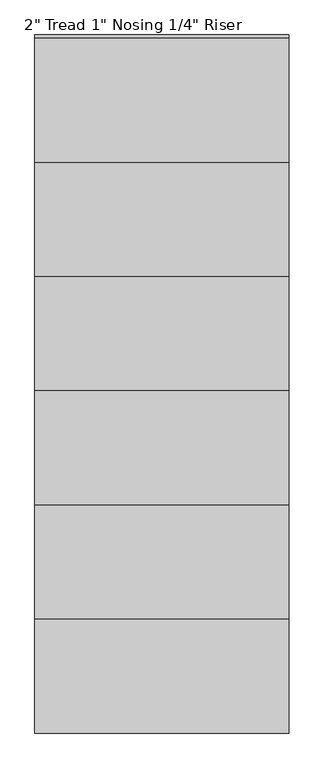
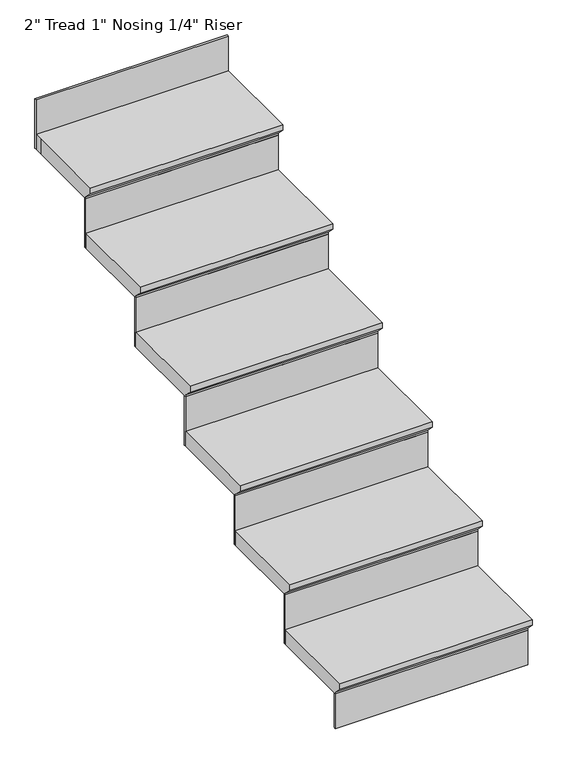
"""IFC4 building model written with IfcOpenShell, lengths in millimetres: stair flight geometry."""

from ifc_helpers import new_model, si_unit, origin, place, context, project, spatial, faceted_brep, source, transform, mapped, element, save


def stair_flight_33de849b(model_context):
    return source(origin(), model_context, "Body", "Brep", [
        faceted_brep([(-912.3629117, -4479.3424149, 150.2833333), (-912.3629117, -4479.3424149, 169.3333333), (-1534.6629117, -4479.3424149, 169.3333333), (-1534.6629117, -4479.3424149, 150.2833333), (-912.3629117, -4453.9424149, 124.8833333), (-1534.6629117, -4453.9424149, 124.8833333), (-912.3629117, -4174.5424149, 169.3333333), (-1534.6629117, -4174.5424149, 169.3333333), (-1534.6629117, -4453.9424149, 118.5333333), (-1534.6629117, -4174.5424149, 118.5333333), (-912.3629117, -4174.5424149, 118.5333333), (-912.3629117, -4453.9424149, 118.5333333)], [[[0, 1, 2, 3]], [[4, 0, 3, 5]], [[2, 1, 6, 7]], [[8, 9, 10, 11]], [[2, 7, 9, 8, 5, 3]], [[8, 11, 4, 5]], [[6, 1, 0, 4, 11, 10]], [[7, 6, 10, 9]]]),
        faceted_brep([(-912.3629117, -4453.9424149, 118.5333333), (-912.3629117, -4453.9424149, 0.0), (-912.3629117, -4447.5924149, 0.0), (-912.3629117, -4447.5924149, 118.5333333), (-1534.6629117, -4453.9424149, 118.5333333), (-1534.6629117, -4447.5924149, 118.5333333), (-1534.6629117, -4447.5924149, 0.0), (-1534.6629117, -4453.9424149, 0.0)], [[[0, 1, 2, 3]], [[4, 5, 6, 7]], [[1, 0, 4, 7]], [[2, 1, 7, 6]], [[3, 2, 6, 5]], [[0, 3, 5, 4]]]),
        faceted_brep([(-912.3629117, -4174.5424149, 287.8666667), (-912.3629117, -4174.5424149, 118.5333333), (-912.3629117, -4168.1924149, 118.5333333), (-912.3629117, -4168.1924149, 287.8666667), (-1534.6629117, -4174.5424149, 287.8666667), (-1534.6629117, -4168.1924149, 287.8666667), (-1534.6629117, -4168.1924149, 118.5333333), (-1534.6629117, -4174.5424149, 118.5333333)], [[[0, 1, 2, 3]], [[4, 5, 6, 7]], [[1, 0, 4, 7]], [[2, 1, 7, 6]], [[3, 2, 6, 5]], [[0, 3, 5, 4]]]),
        faceted_brep([(-1534.6629117, -4199.9424149, 338.6666667), (-912.3629117, -4199.9424149, 338.6666667), (-912.3629117, -3895.1424149, 338.6666667), (-1534.6629117, -3895.1424149, 338.6666667), (-1534.6629117, -4174.5424149, 287.8666667), (-1534.6629117, -3895.1424149, 287.8666667), (-912.3629117, -3895.1424149, 287.8666667), (-912.3629117, -4174.5424149, 287.8666667), (-1534.6629117, -4174.5424149, 294.2166667), (-1534.6629117, -4199.9424149, 319.6166667), (-912.3629117, -4174.5424149, 294.2166667), (-912.3629117, -4199.9424149, 319.6166667)], [[[0, 1, 2, 3]], [[4, 5, 6, 7]], [[0, 3, 5, 4, 8, 9]], [[4, 7, 10, 8]], [[2, 1, 11, 10, 7, 6]], [[3, 2, 6, 5]], [[11, 1, 0, 9]], [[10, 11, 9, 8]]]),
        faceted_brep([(-912.3629117, -3895.1424149, 457.2), (-912.3629117, -3895.1424149, 287.8666667), (-912.3629117, -3888.7924149, 287.8666667), (-912.3629117, -3888.7924149, 457.2), (-1534.6629117, -3895.1424149, 457.2), (-1534.6629117, -3888.7924149, 457.2), (-1534.6629117, -3888.7924149, 287.8666667), (-1534.6629117, -3895.1424149, 287.8666667)], [[[0, 1, 2, 3]], [[4, 5, 6, 7]], [[1, 0, 4, 7]], [[2, 1, 7, 6]], [[3, 2, 6, 5]], [[0, 3, 5, 4]]]),
        faceted_brep([(-1534.6629117, -3920.5424149, 508.0), (-912.3629117, -3920.5424149, 508.0), (-912.3629117, -3615.7424149, 508.0), (-1534.6629117, -3615.7424149, 508.0), (-1534.6629117, -3895.1424149, 457.2), (-1534.6629117, -3615.7424149, 457.2), (-912.3629117, -3615.7424149, 457.2), (-912.3629117, -3895.1424149, 457.2), (-1534.6629117, -3895.1424149, 463.55), (-1534.6629117, -3920.5424149, 488.95), (-912.3629117, -3895.1424149, 463.55), (-912.3629117, -3920.5424149, 488.95)], [[[0, 1, 2, 3]], [[4, 5, 6, 7]], [[0, 3, 5, 4, 8, 9]], [[4, 7, 10, 8]], [[2, 1, 11, 10, 7, 6]], [[3, 2, 6, 5]], [[11, 1, 0, 9]], [[10, 11, 9, 8]]]),
        faceted_brep([(-912.3629117, -3615.7424149, 626.5333333), (-912.3629117, -3615.7424149, 457.2), (-912.3629117, -3609.3924149, 457.2), (-912.3629117, -3609.3924149, 626.5333333), (-1534.6629117, -3615.7424149, 626.5333333), (-1534.6629117, -3609.3924149, 626.5333333), (-1534.6629117, -3609.3924149, 457.2), (-1534.6629117, -3615.7424149, 457.2)], [[[0, 1, 2, 3]], [[4, 5, 6, 7]], [[1, 0, 4, 7]], [[2, 1, 7, 6]], [[3, 2, 6, 5]], [[0, 3, 5, 4]]]),
        faceted_brep([(-1534.6629117, -3641.1424149, 677.3333333), (-912.3629117, -3641.1424149, 677.3333333), (-912.3629117, -3336.3424149, 677.3333333), (-1534.6629117, -3336.3424149, 677.3333333), (-1534.6629117, -3615.7424149, 626.5333333), (-1534.6629117, -3336.3424149, 626.5333333), (-912.3629117, -3336.3424149, 626.5333333), (-912.3629117, -3615.7424149, 626.5333333), (-1534.6629117, -3615.7424149, 632.8833333), (-1534.6629117, -3641.1424149, 658.2833333), (-912.3629117, -3615.7424149, 632.8833333), (-912.3629117, -3641.1424149, 658.2833333)], [[[0, 1, 2, 3]], [[4, 5, 6, 7]], [[0, 3, 5, 4, 8, 9]], [[4, 7, 10, 8]], [[2, 1, 11, 10, 7, 6]], [[3, 2, 6, 5]], [[11, 1, 0, 9]], [[10, 11, 9, 8]]]),
        faceted_brep([(-912.3629117, -3336.3424149, 795.8666667), (-912.3629117, -3336.3424149, 626.5333333), (-912.3629117, -3329.9924149, 626.5333333), (-912.3629117, -3329.9924149, 795.8666667), (-1534.6629117, -3336.3424149, 795.8666667), (-1534.6629117, -3329.9924149, 795.8666667), (-1534.6629117, -3329.9924149, 626.5333333), (-1534.6629117, -3336.3424149, 626.5333333)], [[[0, 1, 2, 3]], [[4, 5, 6, 7]], [[1, 0, 4, 7]], [[2, 1, 7, 6]], [[3, 2, 6, 5]], [[0, 3, 5, 4]]]),
        faceted_brep([(-1534.6629117, -3361.7424149, 846.6666667), (-912.3629117, -3361.7424149, 846.6666667), (-912.3629117, -3056.9424149, 846.6666667), (-1534.6629117, -3056.9424149, 846.6666667), (-1534.6629117, -3336.3424149, 795.8666667), (-1534.6629117, -3056.9424149, 795.8666667), (-912.3629117, -3056.9424149, 795.8666667), (-912.3629117, -3336.3424149, 795.8666667), (-1534.6629117, -3336.3424149, 802.2166667), (-1534.6629117, -3361.7424149, 827.6166667), (-912.3629117, -3336.3424149, 802.2166667), (-912.3629117, -3361.7424149, 827.6166667)], [[[0, 1, 2, 3]], [[4, 5, 6, 7]], [[0, 3, 5, 4, 8, 9]], [[4, 7, 10, 8]], [[2, 1, 11, 10, 7, 6]], [[3, 2, 6, 5]], [[11, 1, 0, 9]], [[10, 11, 9, 8]]]),
        faceted_brep([(-912.3629117, -2777.5424149, 1134.5333333), (-912.3629117, -2777.5424149, 965.2), (-912.3629117, -2771.1924149, 965.2), (-912.3629117, -2771.1924149, 1134.5333333), (-1534.6629117, -2777.5424149, 1134.5333333), (-1534.6629117, -2771.1924149, 1134.5333333), (-1534.6629117, -2771.1924149, 965.2), (-1534.6629117, -2777.5424149, 965.2)], [[[0, 1, 2, 3]], [[4, 5, 6, 7]], [[1, 0, 4, 7]], [[2, 1, 7, 6]], [[3, 2, 6, 5]], [[0, 3, 5, 4]]]),
        faceted_brep([(-912.3629117, -3056.9424149, 965.2), (-912.3629117, -3056.9424149, 795.8666667), (-912.3629117, -3050.5924149, 795.8666667), (-912.3629117, -3050.5924149, 965.2), (-1534.6629117, -3056.9424149, 965.2), (-1534.6629117, -3050.5924149, 965.2), (-1534.6629117, -3050.5924149, 795.8666667), (-1534.6629117, -3056.9424149, 795.8666667)], [[[0, 1, 2, 3]], [[4, 5, 6, 7]], [[1, 0, 4, 7]], [[2, 1, 7, 6]], [[3, 2, 6, 5]], [[0, 3, 5, 4]]]),
        faceted_brep([(-1534.6629117, -2777.5424149, 1016.0), (-1534.6629117, -2802.9424149, 1016.0), (-1534.6629117, -3082.3424149, 1016.0), (-912.3629117, -3082.3424149, 1016.0), (-912.3629117, -2777.5424149, 1016.0), (-1534.6629117, -2802.9424149, 965.2), (-1534.6629117, -2777.5424149, 965.2), (-912.3629117, -2777.5424149, 965.2), (-912.3629117, -3056.9424149, 965.2), (-1534.6629117, -3056.9424149, 965.2), (-1534.6629117, -3056.9424149, 971.55), (-1534.6629117, -3082.3424149, 996.95), (-912.3629117, -3056.9424149, 971.55), (-912.3629117, -3082.3424149, 996.95)], [[[0, 1, 2, 3, 4]], [[5, 6, 7, 8, 9]], [[1, 0, 6, 5]], [[2, 1, 5, 9, 10, 11]], [[9, 8, 12, 10]], [[4, 3, 13, 12, 8, 7]], [[0, 4, 7, 6]], [[13, 3, 2, 11]], [[12, 13, 11, 10]]]),
    ])


if __name__ == "__main__":
    model = new_model("IFC4")
    model_context = context("Model", 3, world=origin())
    ifc_project = project(units=[si_unit("LENGTHUNIT", "METRE", prefix="MILLI")], contexts=[model_context])
    site = spatial("IfcSite", under=ifc_project)
    building = spatial("IfcBuilding", under=site)
    placement = place(None, origin())
    stair_flight_shape = stair_flight_33de849b(model_context)
    element("IfcStairFlight", 1, ObjectType="2\" Tread 1\" Nosing 1/4\" Riser", at=placement, inside=building, context=model_context, shape_type="MappedRepresentation", body=[
        mapped(stair_flight_shape, transform((0.0, 0.0, 0.0), x_axis=(1.0, 0.0, 0.0), y_axis=(0.0, 1.0, 0.0), z_axis=(0.0, 0.0, 1.0))),
    ])
    save(model, "model.ifc")
